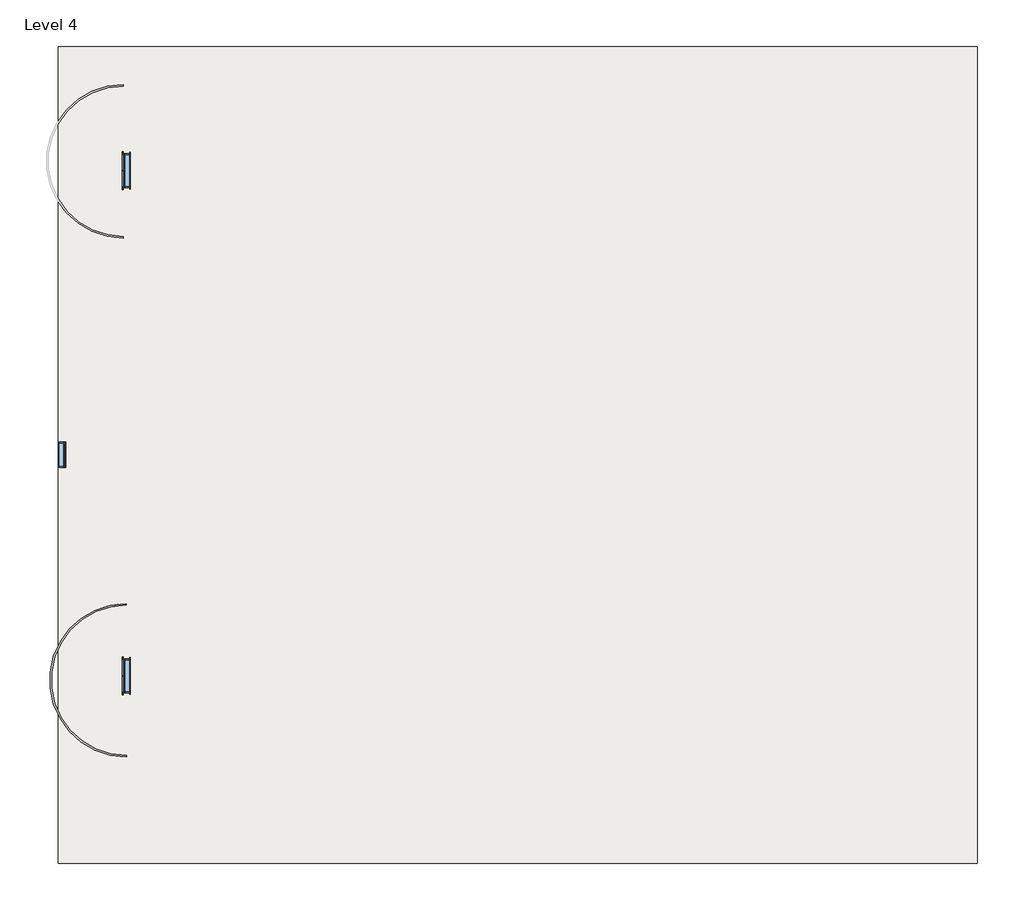
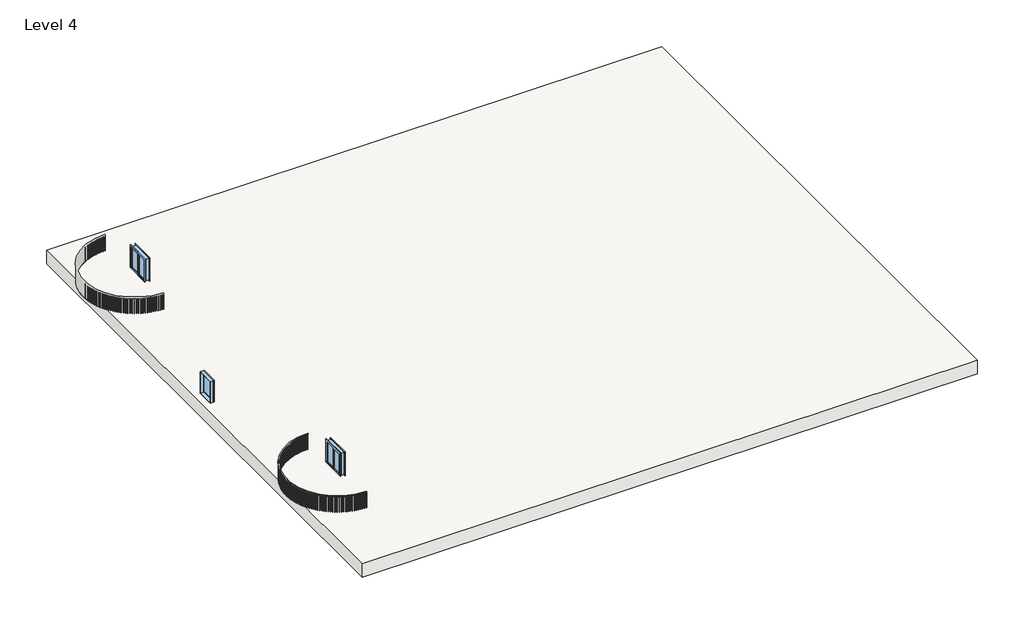
# One storey, part 1 of 2: 3 windows, 1 railing, 1 slab.
"""IFC4 building model written with IfcOpenShell, lengths in millimetres."""

from ifc_helpers import new_model, si_unit, point, frame, frame_2d, origin, place, context, project, spatial, polyline, circle_curve, trimmed, segment, composite_curve, outline, extrude, transform, mapped, element, save
from components import window_534dcd48, window_c1f32544

model = new_model("IFC4")

# Units and contexts
model_context = context("Model", 3, world=origin())
ifc_project = project(units=[si_unit("LENGTHUNIT", "METRE", prefix="MILLI")], contexts=[model_context])

# Site, building, storey
site = spatial("IfcSite", under=ifc_project)
building = spatial("IfcBuilding", under=site)
storey = spatial("IfcBuildingStorey", under=building, Name="Level 4", Elevation=9144.0)

# Railing
placement = place(None, origin())
element("IfcRailing", 1, ObjectType="Handrail - Rectangular", at=placement, inside=storey, context=model_context, shape_type="SweptSolid", body=[
    extrude(outline(composite_curve([segment(trimmed(circle_curve(frame_2d((-15613.8723021, -8267.0443987)), 2743.2), [point((-15613.8723021, -11010.2443987))], [point((-15613.8723021, -5523.8443987))], False, "CARTESIAN"), True, "CONTINUOUS"), segment(polyline([(-15613.8723021, -5523.8443987), (-15613.8723021, -5574.6443987)]), True, "CONTINUOUS"), segment(trimmed(circle_curve(frame_2d((-15613.8723021, -8267.0443987)), 2692.4), [point((-15613.8723021, -5574.6443987))], [point((-15613.8723021, -10959.4443987))], True, "CARTESIAN"), True, "CONTINUOUS"), segment(polyline([(-15613.8723021, -10959.4443987), (-15613.8723021, -11010.2443987)]), True, "CONTINUOUS")], self_intersect=False)), frame((0.0, 0.0, 10007.6), z_axis=(0.0, 0.0, 1.0), x_axis=(1.0, 0.0, 0.0)), (0.0, 0.0, 1.0), 50.8),
    extrude(outline(polyline([(-15627.231195, -10994.3533143), (-15627.2044157, -10975.3033331), (-15608.1544345, -10975.3301124), (-15608.1812138, -10994.3800936), (-15627.231195, -10994.3533143)])), frame((0.0, 0.0, 9144.0), z_axis=(0.0, 0.0, 1.0), x_axis=(1.0, 0.0, 0.0)), (0.0, 0.0, 1.0), 863.6),
    extrude(outline(polyline([(-15729.1535895, -10991.9485449), (-15728.414846, -10972.9128742), (-15709.3791753, -10973.6516178), (-15710.1179188, -10992.6872885), (-15729.1535895, -10991.9485449)])), frame((0.0, 0.0, 9144.0), z_axis=(0.0, 0.0, 1.0), x_axis=(1.0, 0.0, 0.0)), (0.0, 0.0, 1.0), 863.6),
    extrude(outline(polyline([(-15830.914897, -10985.7361601), (-15829.4652214, -10966.7413992), (-15810.4704606, -10968.1910747), (-15811.9201361, -10987.1858356), (-15830.914897, -10985.7361601)])), frame((0.0, 0.0, 9144.0), z_axis=(0.0, 0.0, 1.0), x_axis=(1.0, 0.0, 0.0)), (0.0, 0.0, 1.0), 863.6),
    extrude(outline(polyline([(-15932.3729223, -10975.7248406), (-15930.2143405, -10956.7975316), (-15911.2870315, -10958.9561134), (-15913.4456133, -10977.8834224), (-15932.3729223, -10975.7248406)])), frame((0.0, 0.0, 9144.0), z_axis=(0.0, 0.0, 1.0), x_axis=(1.0, 0.0, 0.0)), (0.0, 0.0, 1.0), 863.6),
    extrude(outline(polyline([(-16033.3858942, -10961.9285757), (-16030.5214224, -10943.0951665), (-16011.6880132, -10945.9596384), (-16014.5524851, -10964.7930475), (-16033.3858942, -10961.9285757)])), frame((0.0, 0.0, 9144.0), z_axis=(0.0, 0.0, 1.0), x_axis=(1.0, 0.0, 0.0)), (0.0, 0.0, 1.0), 863.6),
    extrude(outline(polyline([(-16133.8126634, -10944.3666434), (-16130.2463041, -10925.6534507), (-16111.5331114, -10929.2198099), (-16115.0994706, -10947.9330026), (-16133.8126634, -10944.3666434)])), frame((0.0, 0.0, 9144.0), z_axis=(0.0, 0.0, 1.0), x_axis=(1.0, 0.0, 0.0)), (0.0, 0.0, 1.0), 863.6),
    extrude(outline(polyline([(-16233.5128994, -10923.0635838), (-16229.2496362, -10904.4967562), (-16210.6828086, -10908.7600194), (-16214.9460718, -10927.326847), (-16233.5128994, -10923.0635838)])), frame((0.0, 0.0, 9144.0), z_axis=(0.0, 0.0, 1.0), x_axis=(1.0, 0.0, 0.0)), (0.0, 0.0, 1.0), 863.6),
    extrude(outline(polyline([(-16332.3472874, -10898.0491643), (-16327.3930774, -10879.654646), (-16308.9985591, -10884.608856), (-16313.9527691, -10903.0033743), (-16332.3472874, -10898.0491643)])), frame((0.0, 0.0, 9144.0), z_axis=(0.0, 0.0, 1.0), x_axis=(1.0, 0.0, 0.0)), (0.0, 0.0, 1.0), 863.6),
    extrude(outline(polyline([(-16430.1777221, -10869.3583388), (-16424.5394881, -10851.1618331), (-16406.3429824, -10856.8000671), (-16411.9812164, -10874.9965728), (-16430.1777221, -10869.3583388)])), frame((0.0, 0.0, 9144.0), z_axis=(0.0, 0.0, 1.0), x_axis=(1.0, 0.0, 0.0)), (0.0, 0.0, 1.0), 863.6),
    extrude(outline(polyline([(-16526.8675012, -10837.0311978), (-16520.5531216, -10819.0581316), (-16502.5800554, -10825.3725111), (-16508.8944349, -10843.3455773), (-16526.8675012, -10837.0311978)])), frame((0.0, 0.0, 9144.0), z_axis=(0.0, 0.0, 1.0), x_axis=(1.0, 0.0, 0.0)), (0.0, 0.0, 1.0), 863.6),
    extrude(outline(polyline([(-16622.2815163, -10801.1129136), (-16615.2998146, -10783.3884011), (-16597.5753021, -10790.3701028), (-16604.5570038, -10808.0946153), (-16622.2815163, -10801.1129136)])), frame((0.0, 0.0, 9144.0), z_axis=(0.0, 0.0, 1.0), x_axis=(1.0, 0.0, 0.0)), (0.0, 0.0, 1.0), 863.6),
    extrude(outline(polyline([(-16716.2864416, -10761.653676), (-16708.6471735, -10744.2024845), (-16691.1959821, -10751.8417526), (-16698.8352501, -10769.292944), (-16716.2864416, -10761.653676)])), frame((0.0, 0.0, 9144.0), z_axis=(0.0, 0.0, 1.0), x_axis=(1.0, 0.0, 0.0)), (0.0, 0.0, 1.0), 863.6),
    extrude(outline(polyline([(-16808.7509204, -10718.708623), (-16800.4647607, -10701.5551378), (-16783.3112754, -10709.8412975), (-16791.5974352, -10726.9947828), (-16808.7509204, -10718.708623)])), frame((0.0, 0.0, 9144.0), z_axis=(0.0, 0.0, 1.0), x_axis=(1.0, 0.0, 0.0)), (0.0, 0.0, 1.0), 863.6),
    extrude(outline(polyline([(-16899.5457485, -10672.3377634), (-16890.6242756, -10655.5059536), (-16873.7924658, -10664.4274266), (-16882.7139387, -10681.2592364), (-16899.5457485, -10672.3377634)])), frame((0.0, 0.0, 9144.0), z_axis=(0.0, 0.0, 1.0), x_axis=(1.0, 0.0, 0.0)), (0.0, 0.0, 1.0), 863.6),
    extrude(outline(polyline([(-16988.5440547, -10622.6058931), (-16978.9997349, -10606.1192785), (-16962.5131203, -10615.6635983), (-16972.0574401, -10632.1502129), (-16988.5440547, -10622.6058931)])), frame((0.0, 0.0, 9144.0), z_axis=(0.0, 0.0, 1.0), x_axis=(1.0, 0.0, 0.0)), (0.0, 0.0, 1.0), 863.6),
    extrude(outline(polyline([(-17075.621478, -10569.5825043), (-17065.4676481, -10553.4641223), (-17049.3492661, -10563.6179523), (-17059.5030961, -10579.7363343), (-17075.621478, -10569.5825043)])), frame((0.0, 0.0, 9144.0), z_axis=(0.0, 0.0, 1.0), x_axis=(1.0, 0.0, 0.0)), (0.0, 0.0, 1.0), 863.6),
    extrude(outline(polyline([(-17160.656342, -10513.3416887), (-17149.9071902, -10497.6140622), (-17134.1795637, -10508.363214), (-17144.9287154, -10524.0908405), (-17160.656342, -10513.3416887)])), frame((0.0, 0.0, 9144.0), z_axis=(0.0, 0.0, 1.0), x_axis=(1.0, 0.0, 0.0)), (0.0, 0.0, 1.0), 863.6),
    extrude(outline(polyline([(-17243.5298239, -10453.9620338), (-17232.2003705, -10438.6471396), (-17216.8854763, -10449.976593), (-17228.2149296, -10465.2914872), (-17243.5298239, -10453.9620338)])), frame((0.0, 0.0, 9144.0), z_axis=(0.0, 0.0, 1.0), x_axis=(1.0, 0.0, 0.0)), (0.0, 0.0, 1.0), 863.6),
    extrude(outline(polyline([(-17324.1261214, -10391.5265132), (-17312.2321975, -10376.6457513), (-17297.3514357, -10388.5396752), (-17309.2453596, -10403.4204371), (-17324.1261214, -10391.5265132)])), frame((0.0, 0.0, 9144.0), z_axis=(0.0, 0.0, 1.0), x_axis=(1.0, 0.0, 0.0)), (0.0, 0.0, 1.0), 863.6),
    extrude(outline(polyline([(-17402.3326143, -10326.1223703), (-17389.8908397, -10311.6965343), (-17375.4650036, -10324.1383088), (-17387.9067782, -10338.5641449), (-17402.3326143, -10326.1223703)])), frame((0.0, 0.0, 9144.0), z_axis=(0.0, 0.0, 1.0), x_axis=(1.0, 0.0, 0.0)), (0.0, 0.0, 1.0), 863.6),
    extrude(outline(polyline([(-17478.0400213, -10257.840997), (-17465.0677814, -10243.8902446), (-17451.117029, -10256.8624845), (-17464.0892689, -10270.8132369), (-17478.0400213, -10257.840997)])), frame((0.0, 0.0, 9144.0), z_axis=(0.0, 0.0, 1.0), x_axis=(1.0, 0.0, 0.0)), (0.0, 0.0, 1.0), 863.6),
    extrude(outline(polyline([(-17551.1425537, -10186.7778056), (-17537.6579752, -10173.3216307), (-17524.2018003, -10186.8062093), (-17537.6863789, -10200.2623841), (-17551.1425537, -10186.7778056)])), frame((0.0, 0.0, 9144.0), z_axis=(0.0, 0.0, 1.0), x_axis=(1.0, 0.0, 0.0)), (0.0, 0.0, 1.0), 863.6),
    extrude(outline(polyline([(-17621.5380624, -10113.0320953), (-17607.5599877, -10100.0893009), (-17594.6171933, -10114.0673756), (-17608.595268, -10127.01017), (-17621.5380624, -10113.0320953)])), frame((0.0, 0.0, 9144.0), z_axis=(0.0, 0.0, 1.0), x_axis=(1.0, 0.0, 0.0)), (0.0, 0.0, 1.0), 863.6),
    extrude(outline(polyline([(-17689.128181, -10036.7069141), (-17674.6761422, -10024.2955856), (-17662.2648137, -10038.7476243), (-17676.7168525, -10051.1589528), (-17689.128181, -10036.7069141)])), frame((0.0, 0.0, 9144.0), z_axis=(0.0, 0.0, 1.0), x_axis=(1.0, 0.0, 0.0)), (0.0, 0.0, 1.0), 863.6),
    extrude(outline(polyline([(-17753.8184631, -9957.908914), (-17738.9126547, -9946.0463942), (-17727.0501349, -9960.9522026), (-17741.9559433, -9972.8147224), (-17753.8184631, -9957.908914)])), frame((0.0, 0.0, 9144.0), z_axis=(0.0, 0.0, 1.0), x_axis=(1.0, 0.0, 0.0)), (0.0, 0.0, 1.0), 863.6),
    extrude(outline(polyline([(-17815.5185146, -9876.7482026), (-17800.179765, -9865.4510675), (-17788.8826299, -9880.789817), (-17804.2213795, -9892.0869522), (-17815.5185146, -9876.7482026)])), frame((0.0, 0.0, 9144.0), z_axis=(0.0, 0.0, 1.0), x_axis=(1.0, 0.0, 0.0)), (0.0, 0.0, 1.0), 863.6),
    extrude(outline(polyline([(-17874.1421194, -9793.338189), (-17858.3918621, -9782.6222244), (-17847.6758976, -9798.3724817), (-17863.4261549, -9809.0884462), (-17874.1421194, -9793.338189)])), frame((0.0, 0.0, 9144.0), z_axis=(0.0, 0.0, 1.0), x_axis=(1.0, 0.0, 0.0)), (0.0, 0.0, 1.0), 863.6),
    extrude(outline(polyline([(-17929.6073606, -9707.7954251), (-17913.467604, -9697.6756051), (-17903.347784, -9713.8153616), (-17919.4875405, -9723.9351817), (-17929.6073606, -9707.7954251)])), frame((0.0, 0.0, 9144.0), z_axis=(0.0, 0.0, 1.0), x_axis=(1.0, 0.0, 0.0)), (0.0, 0.0, 1.0), 863.6),
    extrude(outline(polyline([(-17981.8367343, -9620.2394434), (-17965.3300312, -9610.7299086), (-17955.8204964, -9627.2366117), (-17972.3271995, -9636.7461465), (-17981.8367343, -9620.2394434)])), frame((0.0, 0.0, 9144.0), z_axis=(0.0, 0.0, 1.0), x_axis=(1.0, 0.0, 0.0)), (0.0, 0.0, 1.0), 863.6),
    extrude(outline(polyline([(-18030.7572585, -9530.7925891), (-18013.9066743, -9521.9066277), (-18005.0207128, -9538.7572119), (-18021.871297, -9547.6431733), (-18030.7572585, -9530.7925891)])), frame((0.0, 0.0, 9144.0), z_axis=(0.0, 0.0, 1.0), x_axis=(1.0, 0.0, 0.0)), (0.0, 0.0, 1.0), 863.6),
    extrude(outline(polyline([(-18076.3005745, -9439.5798499), (-18059.1296552, -9431.3298785), (-18050.8796837, -9448.5007978), (-18068.0506031, -9456.7507693), (-18076.3005745, -9439.5798499)])), frame((0.0, 0.0, 9144.0), z_axis=(0.0, 0.0, 1.0), x_axis=(1.0, 0.0, 0.0)), (0.0, 0.0, 1.0), 863.6),
    extrude(outline(polyline([(-18118.4030429, -9346.728681), (-18100.9357821, -9339.1262276), (-18093.3333287, -9356.5934885), (-18110.8005895, -9364.1959419), (-18118.4030429, -9346.728681)])), frame((0.0, 0.0, 9144.0), z_axis=(0.0, 0.0, 1.0), x_axis=(1.0, 0.0, 0.0)), (0.0, 0.0, 1.0), 863.6),
    extrude(outline(polyline([(-18157.0058323, -9252.3688268), (-18139.2666376, -9245.4245147), (-18132.3223254, -9263.1637094), (-18150.0615201, -9270.1080215), (-18157.0058323, -9252.3688268)])), frame((0.0, 0.0, 9144.0), z_axis=(0.0, 0.0, 1.0), x_axis=(1.0, 0.0, 0.0)), (0.0, 0.0, 1.0), 863.6),
    extrude(outline(polyline([(-18192.0550015, -9156.6321402), (-18174.0686606, -9150.3556729), (-18167.7921932, -9168.3420137), (-18185.7785341, -9174.6184811), (-18192.0550015, -9156.6321402)])), frame((0.0, 0.0, 9144.0), z_axis=(0.0, 0.0, 1.0), x_axis=(1.0, 0.0, 0.0)), (0.0, 0.0, 1.0), 863.6),
    extrude(outline(polyline([(-18223.5015748, -9059.6523978), (-18205.2932208, -9054.0525456), (-18199.6933686, -9072.2608996), (-18217.9017226, -9077.8607518), (-18223.5015748, -9059.6523978)])), frame((0.0, 0.0, 9144.0), z_axis=(0.0, 0.0, 1.0), x_axis=(1.0, 0.0, 0.0)), (0.0, 0.0, 1.0), 863.6),
    extrude(outline(polyline([(-18251.3016108, -8961.5651131), (-18232.8966869, -8956.6497009), (-18227.9812748, -8975.0546248), (-18246.3861986, -8979.970037), (-18251.3016108, -8961.5651131)])), frame((0.0, 0.0, 9144.0), z_axis=(0.0, 0.0, 1.0), x_axis=(1.0, 0.0, 0.0)), (0.0, 0.0, 1.0), 863.6),
    extrude(outline(polyline([(-18275.4162634, -8862.5073473), (-18256.8404876, -8858.2832437), (-18252.6163839, -8876.8590196), (-18271.1921598, -8881.0831232), (-18275.4162634, -8862.5073473)])), frame((0.0, 0.0, 9144.0), z_axis=(0.0, 0.0, 1.0), x_axis=(1.0, 0.0, 0.0)), (0.0, 0.0, 1.0), 863.6),
    extrude(outline(polyline([(-18295.8118362, -8762.6175179), (-18277.0911651, -8759.0906253), (-18273.5642725, -8777.8112965), (-18292.2849436, -8781.338189), (-18295.8118362, -8762.6175179)])), frame((0.0, 0.0, 9144.0), z_axis=(0.0, 0.0, 1.0), x_axis=(1.0, 0.0, 0.0)), (0.0, 0.0, 1.0), 863.6),
    extrude(outline(polyline([(-18312.4598298, -8662.0352047), (-18293.6204224, -8659.2104514), (-18290.7956691, -8678.0498587), (-18309.6350765, -8680.874612), (-18312.4598298, -8662.0352047)])), frame((0.0, 0.0, 9144.0), z_axis=(0.0, 0.0, 1.0), x_axis=(1.0, 0.0, 0.0)), (0.0, 0.0, 1.0), 863.6),
    extrude(outline(polyline([(-18325.3369811, -8560.9009553), (-18306.4051626, -8558.7822885), (-18304.2864958, -8577.714107), (-18323.2183143, -8579.8327738), (-18325.3369811, -8560.9009553)])), frame((0.0, 0.0, 9144.0), z_axis=(0.0, 0.0, 1.0), x_axis=(1.0, 0.0, 0.0)), (0.0, 0.0, 1.0), 863.6),
    extrude(outline(polyline([(-18334.4252965, -8459.3560886), (-18315.427521, -8457.9464688), (-18314.0179011, -8476.9442442), (-18333.0156766, -8478.3538641), (-18334.4252965, -8459.3560886)])), frame((0.0, 0.0, 9144.0), z_axis=(0.0, 0.0, 1.0), x_axis=(1.0, 0.0, 0.0)), (0.0, 0.0, 1.0), 863.6),
    extrude(outline(polyline([(-18339.7120764, -8357.5424973), (-18320.6748904, -8356.8438941), (-18319.9762872, -8375.8810802), (-18339.0134732, -8376.5796834), (-18339.7120764, -8357.5424973)])), frame((0.0, 0.0, 9144.0), z_axis=(0.0, 0.0, 1.0), x_axis=(1.0, 0.0, 0.0)), (0.0, 0.0, 1.0), 863.6),
    extrude(outline(polyline([(-18341.1899336, -8255.6024494), (-18322.1399383, -8255.6158391), (-18322.1533279, -8274.6658344), (-18341.2033232, -8274.6524447), (-18341.1899336, -8255.6024494)])), frame((0.0, 0.0, 9144.0), z_axis=(0.0, 0.0, 1.0), x_axis=(1.0, 0.0, 0.0)), (0.0, 0.0, 1.0), 863.6),
    extrude(outline(polyline([(-18338.8568028, -8153.6783898), (-18319.8206176, -8154.4037536), (-18320.5459814, -8173.4399388), (-18339.5821666, -8172.7145751), (-18338.8568028, -8153.6783898)])), frame((0.0, 0.0, 9144.0), z_axis=(0.0, 0.0, 1.0), x_axis=(1.0, 0.0, 0.0)), (0.0, 0.0, 1.0), 863.6),
    extrude(outline(polyline([(-18332.7159444, -8051.912741), (-18313.7201692, -8053.3490654), (-18315.1564936, -8072.3448405), (-18334.1522687, -8070.9085161), (-18332.7159444, -8051.912741)])), frame((0.0, 0.0, 9144.0), z_axis=(0.0, 0.0, 1.0), x_axis=(1.0, 0.0, 0.0)), (0.0, 0.0, 1.0), 863.6),
    extrude(outline(polyline([(-18322.775939, -7950.4477041), (-18303.8471175, -7952.592982), (-18305.9923954, -7971.5218035), (-18324.9212169, -7969.3765256), (-18322.775939, -7950.4477041)])), frame((0.0, 0.0, 9144.0), z_axis=(0.0, 0.0, 1.0), x_axis=(1.0, 0.0, 0.0)), (0.0, 0.0, 1.0), 863.6),
    extrude(outline(polyline([(-18309.0506764, -7849.4250602), (-18290.2152585, -7852.2762939), (-18293.0664923, -7871.1117118), (-18311.9019101, -7868.260478), (-18309.0506764, -7849.4250602)])), frame((0.0, 0.0, 9144.0), z_axis=(0.0, 0.0, 1.0), x_axis=(1.0, 0.0, 0.0)), (0.0, 0.0, 1.0), 863.6),
    extrude(outline(polyline([(-18291.5593353, -7748.9859721), (-18272.8436405, -7752.5391776), (-18276.396846, -7771.2548723), (-18295.1125408, -7767.7016669), (-18291.5593353, -7748.9859721)])), frame((0.0, 0.0, 9144.0), z_axis=(0.0, 0.0, 1.0), x_axis=(1.0, 0.0, 0.0)), (0.0, 0.0, 1.0), 863.6),
    extrude(outline(polyline([(-18270.3263571, -7649.2707874), (-18251.7565376, -7653.5209995), (-18256.0067497, -7672.0908191), (-18274.5765692, -7667.8406069), (-18270.3263571, -7649.2707874)])), frame((0.0, 0.0, 9144.0), z_axis=(0.0, 0.0, 1.0), x_axis=(1.0, 0.0, 0.0)), (0.0, 0.0, 1.0), 863.6),
    extrude(outline(polyline([(-18245.3814115, -7550.418842), (-18226.9834156, -7555.3601218), (-18231.9246954, -7573.7581178), (-18250.3226913, -7568.816838), (-18245.3814115, -7550.418842)])), frame((0.0, 0.0, 9144.0), z_axis=(0.0, 0.0, 1.0), x_axis=(1.0, 0.0, 0.0)), (0.0, 0.0, 1.0), 863.6),
    extrude(outline(polyline([(-18216.7593549, -7452.5682656), (-18198.5588909, -7458.1937085), (-18204.1843337, -7476.3941726), (-18222.3847978, -7470.7687297), (-18216.7593549, -7452.5682656)])), frame((0.0, 0.0, 9144.0), z_axis=(0.0, 0.0, 1.0), x_axis=(1.0, 0.0, 0.0)), (0.0, 0.0, 1.0), 863.6),
    extrude(outline(polyline([(-18184.5001822, -7355.8557887), (-18166.5226822, -7362.1575339), (-18172.8244275, -7380.1350339), (-18190.8019275, -7373.8332887), (-18184.5001822, -7355.8557887)])), frame((0.0, 0.0, 9144.0), z_axis=(0.0, 0.0, 1.0), x_axis=(1.0, 0.0, 0.0)), (0.0, 0.0, 1.0), 863.6),
    extrude(outline(polyline([(-18148.6489704, -7260.4165513), (-18130.9195551, -7267.3857933), (-18137.888797, -7285.1152086), (-18155.6182123, -7278.1459666), (-18148.6489704, -7260.4165513)])), frame((0.0, 0.0, 9144.0), z_axis=(0.0, 0.0, 1.0), x_axis=(1.0, 0.0, 0.0)), (0.0, 0.0, 1.0), 863.6),
    extrude(outline(polyline([(-18109.2558157, -7166.3839145), (-18091.7992591, -7174.0109148), (-18099.4262594, -7191.4674713), (-18116.8828159, -7183.8404711), (-18109.2558157, -7166.3839145)])), frame((0.0, 0.0, 9144.0), z_axis=(0.0, 0.0, 1.0), x_axis=(1.0, 0.0, 0.0)), (0.0, 0.0, 1.0), 863.6),
    extrude(outline(polyline([(-18066.3757637, -7073.8892738), (-18049.2164586, -7082.1633749), (-18057.4905597, -7099.32268), (-18074.6498648, -7091.0485789), (-18066.3757637, -7073.8892738)])), frame((0.0, 0.0, 9144.0), z_axis=(0.0, 0.0, 1.0), x_axis=(1.0, 0.0, 0.0)), (0.0, 0.0, 1.0), 863.6),
    extrude(outline(polyline([(-18020.0687324, -6983.0618755), (-18003.2306562, -6991.9715157), (-18012.1402963, -7008.8095919), (-18028.9783726, -6999.8999518), (-18020.0687324, -6983.0618755)])), frame((0.0, 0.0, 9144.0), z_axis=(0.0, 0.0, 1.0), x_axis=(1.0, 0.0, 0.0)), (0.0, 0.0, 1.0), 863.6),
    extrude(outline(polyline([(-17970.3994285, -6894.0286364), (-17953.9061096, -6903.5613658), (-17963.4388391, -6920.0546848), (-17979.932158, -6910.5219553), (-17970.3994285, -6894.0286364)])), frame((0.0, 0.0, 9144.0), z_axis=(0.0, 0.0, 1.0), x_axis=(1.0, 0.0, 0.0)), (0.0, 0.0, 1.0), 863.6),
    extrude(outline(polyline([(-17917.4372568, -6806.913966), (-17901.311742, -6817.0564643), (-17911.4542403, -6833.1819791), (-17927.5797552, -6823.0394808), (-17917.4372568, -6806.913966)])), frame((0.0, 0.0, 9144.0), z_axis=(0.0, 0.0, 1.0), x_axis=(1.0, 0.0, 0.0)), (0.0, 0.0, 1.0), 863.6),
    extrude(outline(polyline([(-17861.2562235, -6721.8395932), (-17845.5210456, -6732.5776878), (-17856.2591402, -6748.3128657), (-17871.9943181, -6737.5747711), (-17861.2562235, -6721.8395932)])), frame((0.0, 0.0, 9144.0), z_axis=(0.0, 0.0, 1.0), x_axis=(1.0, 0.0, 0.0)), (0.0, 0.0, 1.0), 863.6),
    extrude(outline(polyline([(-17801.9348324, -6638.9243956), (-17786.6119788, -6650.2430818), (-17797.9306651, -6665.5659354), (-17813.2535187, -6654.2472492), (-17801.9348324, -6638.9243956)])), frame((0.0, 0.0, 9144.0), z_axis=(0.0, 0.0, 1.0), x_axis=(1.0, 0.0, 0.0)), (0.0, 0.0, 1.0), 863.6),
    extrude(outline(polyline([(-17739.5559758, -6558.284234), (-17724.6668577, -6570.1676957), (-17736.5503195, -6585.0568138), (-17751.4394375, -6573.1733521), (-17739.5559758, -6558.284234)])), frame((0.0, 0.0, 9144.0), z_axis=(0.0, 0.0, 1.0), x_axis=(1.0, 0.0, 0.0)), (0.0, 0.0, 1.0), 863.6),
    extrude(outline(polyline([(-17674.206818, -6480.03179), (-17659.7722406, -6492.463422), (-17672.2038726, -6506.8979994), (-17686.63845, -6494.4663674), (-17674.206818, -6480.03179)])), frame((0.0, 0.0, 9144.0), z_axis=(0.0, 0.0, 1.0), x_axis=(1.0, 0.0, 0.0)), (0.0, 0.0, 1.0), 863.6),
    extrude(outline(polyline([(-17605.978674, -6404.2764087), (-17592.0188072, -6417.2388399), (-17604.9812384, -6431.1987066), (-17618.9411051, -6418.2362755), (-17605.978674, -6404.2764087)])), frame((0.0, 0.0, 9144.0), z_axis=(0.0, 0.0, 1.0), x_axis=(1.0, 0.0, 0.0)), (0.0, 0.0, 1.0), 863.6),
    extrude(outline(polyline([(-17534.9668816, -6331.1239463), (-17521.5012322, -6344.5990636), (-17534.9763495, -6358.064713), (-17548.4419989, -6344.5895957), (-17534.9668816, -6331.1239463)])), frame((0.0, 0.0, 9144.0), z_axis=(0.0, 0.0, 1.0), x_axis=(1.0, 0.0, 0.0)), (0.0, 0.0, 1.0), 863.6),
    extrude(outline(polyline([(-17461.2706683, -6260.6766214), (-17448.3180524, -6274.6455956), (-17462.2870265, -6287.5982116), (-17475.2396425, -6273.6292374), (-17461.2706683, -6260.6766214)])), frame((0.0, 0.0, 9144.0), z_axis=(0.0, 0.0, 1.0), x_axis=(1.0, 0.0, 0.0)), (0.0, 0.0, 1.0), 863.6),
    extrude(outline(polyline([(-17384.9930129, -6193.032873), (-17372.5715296, -6207.4761846), (-17387.0148412, -6219.897668), (-17399.4363246, -6205.4543563), (-17384.9930129, -6193.032873)])), frame((0.0, 0.0, 9144.0), z_axis=(0.0, 0.0, 1.0), x_axis=(1.0, 0.0, 0.0)), (0.0, 0.0, 1.0), 863.6),
    extrude(outline(polyline([(-17306.2405011, -6128.2872222), (-17294.3675074, -6143.1846891), (-17309.2649743, -6155.0576828), (-17321.137968, -6140.1602159), (-17306.2405011, -6128.2872222)])), frame((0.0, 0.0, 9144.0), z_axis=(0.0, 0.0, 1.0), x_axis=(1.0, 0.0, 0.0)), (0.0, 0.0, 1.0), 863.6),
    extrude(outline(polyline([(-17225.1231768, -6066.5301406), (-17213.8152633, -6081.860946), (-17229.1460687, -6093.1688594), (-17240.4539822, -6077.8380541), (-17225.1231768, -6066.5301406)])), frame((0.0, 0.0, 9144.0), z_axis=(0.0, 0.0, 1.0), x_axis=(1.0, 0.0, 0.0)), (0.0, 0.0, 1.0), 863.6),
    extrude(outline(polyline([(-17141.7543884, -6007.847924), (-17131.0273562, -6023.5906455), (-17146.7700777, -6034.3176777), (-17157.4971099, -6018.5749562), (-17141.7543884, -6007.847924)])), frame((0.0, 0.0, 9144.0), z_axis=(0.0, 0.0, 1.0), x_axis=(1.0, 0.0, 0.0)), (0.0, 0.0, 1.0), 863.6),
    extrude(outline(polyline([(-17056.2506305, -5952.3225712), (-17046.1194688, -5968.4552108), (-17062.2521085, -5978.5863725), (-17072.3832702, -5962.4537328), (-17056.2506305, -5952.3225712)])), frame((0.0, 0.0, 9144.0), z_axis=(0.0, 0.0, 1.0), x_axis=(1.0, 0.0, 0.0)), (0.0, 0.0, 1.0), 863.6),
    extrude(outline(polyline([(-16968.7313808, -5900.03167), (-16959.2102463, -5916.5316851), (-16975.7102614, -5926.0528195), (-16985.2313959, -5909.5528044), (-16968.7313808, -5900.03167)])), frame((0.0, 0.0, 9144.0), z_axis=(0.0, 0.0, 1.0), x_axis=(1.0, 0.0, 0.0)), (0.0, 0.0, 1.0), 863.6),
    extrude(outline(polyline([(-16879.3189333, -5851.0482885), (-16870.4211303, -5867.8926229), (-16887.2654647, -5876.7904259), (-16896.1632677, -5859.9460915), (-16879.3189333, -5851.0482885)])), frame((0.0, 0.0, 9144.0), z_axis=(0.0, 0.0, 1.0), x_axis=(1.0, 0.0, 0.0)), (0.0, 0.0, 1.0), 863.6),
    extrude(outline(polyline([(-16788.1382277, -5805.4408731), (-16779.8761894, -5822.6059896), (-16797.0413058, -5830.8680279), (-16805.3033441, -5813.7029114), (-16788.1382277, -5805.4408731)])), frame((0.0, 0.0, 9144.0), z_axis=(0.0, 0.0, 1.0), x_axis=(1.0, 0.0, 0.0)), (0.0, 0.0, 1.0), 863.6),
    extrude(outline(polyline([(-16695.3166742, -5763.2731529), (-16687.7019455, -5780.7350659), (-16705.1638585, -5788.3497946), (-16712.7785872, -5770.8878816), (-16695.3166742, -5763.2731529)])), frame((0.0, 0.0, 9144.0), z_axis=(0.0, 0.0, 1.0), x_axis=(1.0, 0.0, 0.0)), (0.0, 0.0, 1.0), 863.6),
    extrude(outline(polyline([(-16600.983976, -5724.6040505), (-16594.0271973, -5742.3383598), (-16611.7615066, -5749.2951386), (-16618.7182854, -5731.5608292), (-16600.983976, -5724.6040505)])), frame((0.0, 0.0, 9144.0), z_axis=(0.0, 0.0, 1.0), x_axis=(1.0, 0.0, 0.0)), (0.0, 0.0, 1.0), 863.6),
    extrude(outline(polyline([(-16505.271948, -5689.4875996), (-16498.9828402, -5707.4695245), (-16516.9647651, -5713.7586324), (-16523.2538729, -5695.7767075), (-16505.271948, -5689.4875996)])), frame((0.0, 0.0, 9144.0), z_axis=(0.0, 0.0, 1.0), x_axis=(1.0, 0.0, 0.0)), (0.0, 0.0, 1.0), 863.6),
    extrude(outline(polyline([(-16408.3143324, -5657.97287), (-16402.7016834, -5676.1772836), (-16420.906097, -5681.7899325), (-16426.5187459, -5663.5855189), (-16408.3143324, -5657.97287)])), frame((0.0, 0.0, 9144.0), z_axis=(0.0, 0.0, 1.0), x_axis=(1.0, 0.0, 0.0)), (0.0, 0.0, 1.0), 863.6),
    extrude(outline(polyline([(-16310.2466117, -5630.1038984), (-16305.3182645, -5648.5053628), (-16323.7197289, -5653.43371), (-16328.6480761, -5635.0322456), (-16310.2466117, -5630.1038984)])), frame((0.0, 0.0, 9144.0), z_axis=(0.0, 0.0, 1.0), x_axis=(1.0, 0.0, 0.0)), (0.0, 0.0, 1.0), 863.6),
    extrude(outline(polyline([(-16211.2058198, -5605.9196271), (-16206.9686609, -5624.4924294), (-16225.5414632, -5628.7295883), (-16229.7786221, -5610.1567861), (-16211.2058198, -5605.9196271)])), frame((0.0, 0.0, 9144.0), z_axis=(0.0, 0.0, 1.0), x_axis=(1.0, 0.0, 0.0)), (0.0, 0.0, 1.0), 863.6),
    extrude(outline(polyline([(-16111.3303505, -5585.4538499), (-16107.7903006, -5604.1720375), (-16126.5084882, -5607.7120874), (-16130.048538, -5588.9938998), (-16111.3303505, -5585.4538499)])), frame((0.0, 0.0, 9144.0), z_axis=(0.0, 0.0, 1.0), x_axis=(1.0, 0.0, 0.0)), (0.0, 0.0, 1.0), 863.6),
    extrude(outline(polyline([(-16010.7597634, -5568.7351643), (-16007.9217692, -5587.5725816), (-16026.7591865, -5590.4105758), (-16029.5971807, -5571.5731585), (-16010.7597634, -5568.7351643)])), frame((0.0, 0.0, 9144.0), z_axis=(0.0, 0.0, 1.0), x_axis=(1.0, 0.0, 0.0)), (0.0, 0.0, 1.0), 863.6),
    extrude(outline(polyline([(-15909.63459, -5555.7869321), (-15907.5026171, -5574.7172567), (-15926.4329418, -5576.8492296), (-15928.5649146, -5557.918905), (-15909.63459, -5555.7869321)])), frame((0.0, 0.0, 9144.0), z_axis=(0.0, 0.0, 1.0), x_axis=(1.0, 0.0, 0.0)), (0.0, 0.0, 1.0), 863.6),
    extrude(outline(polyline([(-15808.0961363, -5546.6272462), (-15806.6731638, -5565.6240262), (-15825.6699438, -5567.0469987), (-15827.0929163, -5548.0502187), (-15808.0961363, -5546.6272462)])), frame((0.0, 0.0, 9144.0), z_axis=(0.0, 0.0, 1.0), x_axis=(1.0, 0.0, 0.0)), (0.0, 0.0, 1.0), 863.6),
    extrude(outline(polyline([(-15706.286286, -5541.268906), (-15705.5743024, -5560.3055963), (-15724.6109927, -5561.01758), (-15725.3229764, -5541.9808896), (-15706.286286, -5541.268906)])), frame((0.0, 0.0, 9144.0), z_axis=(0.0, 0.0, 1.0), x_axis=(1.0, 0.0, 0.0)), (0.0, 0.0, 1.0), 863.6),
    extrude(outline(polyline([(-15632.955606, -10994.3192673), (-15632.8888422, -10975.2693843), (-15613.8389591, -10975.3361482), (-15613.905723, -10994.3860312), (-15632.955606, -10994.3192673)])), frame((0.0, 0.0, 9144.0), z_axis=(0.0, 0.0, 1.0), x_axis=(1.0, 0.0, 0.0)), (0.0, 0.0, 1.0), 863.6),
    extrude(outline(polyline([(-15613.905723, -5539.7027662), (-15613.8389591, -5558.7526493), (-15632.8888422, -5558.8194131), (-15632.955606, -5539.7695301), (-15613.905723, -5539.7027662)])), frame((0.0, 0.0, 9144.0), z_axis=(0.0, 0.0, 1.0), x_axis=(1.0, 0.0, 0.0)), (0.0, 0.0, 1.0), 863.6),
])

# Slab
element("IfcSlab", 2, ObjectType="Generic - 12\"", at=placement, inside=storey, context=model_context, shape_type="SweptSolid", body=[
    extrude(outline(polyline([(14866.1276979, 14440.5556013), (14866.1276979, -14820.2443987), (-18052.2723021, -14820.2443987), (-18052.2723021, 14440.5556013), (14866.1276979, 14440.5556013)])), frame((0.0, 0.0, 8382.0), z_axis=(0.0, 0.0, 1.0), x_axis=(1.0, 0.0, 0.0)), (0.0, 0.0, 1.0), 762.0),
])

# Windows
window_shape = window_534dcd48(model_context)
element("IfcWindow", 3, ObjectType="Casement Dbl with Trim : 48\" x 48\"", at=placement, inside=storey, context=model_context, shape_type="MappedRepresentation", body=[
    mapped(window_shape, transform((-15594.8223021, 9995.5556013, 8737.1054136), x_axis=(0.0, 1.0, 0.0), y_axis=(-1.0, 0.0, 0.0), z_axis=(0.0, 0.0, 1.0))),
])
element("IfcWindow", 4, ObjectType="Casement Dbl with Trim : 48\" x 48\"", at=placement, inside=storey, context=model_context, shape_type="MappedRepresentation", body=[
    mapped(window_shape, transform((-15594.8223021, -8114.6443987, 8725.1499872), x_axis=(0.0, 1.0, 0.0), y_axis=(-1.0, 0.0, 0.0), z_axis=(0.0, 0.0, 1.0))),
])
window_2_shape = window_c1f32544(model_context)
element("IfcWindow", 5, ObjectType="Fixed : 36\" x 48\"", at=placement, inside=storey, context=model_context, shape_type="MappedRepresentation", body=[
    mapped(window_2_shape, transform((-17899.8723021, -227.9443987, 8721.0470019), x_axis=(0.0, -1.0, 0.0), y_axis=(1.0, 0.0, 0.0), z_axis=(0.0, 0.0, 1.0))),
])

save(model, "model.ifc")

# Revit data of these elements
# Type "Handrail - Rectangular"
#   Assembly Code = "C2010400"
#   built-in parameter 1008612 = 0.0416667 (stored number, unit not read)
#   built-in parameter 1008611 = 0.0416667 (stored number, unit not read)
#   built-in parameter 1008609 = 0.333333 (stored number, unit not read)
#   built-in parameter 1008604 = 0.166667 (stored number, unit not read)
#   built-in parameter 1008603 = 0.166667 (stored number, unit not read)
#   Railing Height = 3' - 0"
#   built-in parameter 1008630 = 2
#   built-in parameter 1008610 = 2
#   built-in parameter 1008618 = Baluster - Square : 3/4"
# Type "Generic - 12\""
#   Assembly Code = "B1010"
#   Function = 0
#   Layers, outside or top first: 2' - 6" no material (function 1)
# Type "Casement Dbl with Trim : 48\" x 48\""
#   Type Mark = "19"
#   Construction Type Id = "GSP4R"
#   Assembly Code = "B2020100"
#   Analytic Construction = "1/8 in Pilkington single glazing"
#   Visual Light Transmittance = 0.9
#   Solar Heat Gain Coefficient = 0.78
#   Heat Transfer Coefficient (U) = 0.6496 BTU/(h·ft²·°F)
#   Height = 4' - 0"
#   Default Sill Height = 3' - 0"
#   Trim Projection - Ext. = 0' - 0 1/2"
#   Trim Projection - Int. = 0' - 0 3/4"
#   Trim Width - Exterior = 0' - 3 1/2"
#   Trim Width - Interior = 0' - 3 1/2"
#   Width = 4' - 0"
#   Window Inset = 0' - 0 3/4"
#   Define Thermal Properties by = 1
#   Glass Pane Material = Glass
#   Sash Material = Sash
#   Trim Exterior Material = Trim
#   Trim Interior Material = Trim
#   Wall Closure = (empty or 0)
# Type "Fixed : 36\" x 48\""
#   Type Mark = "1"
#   Construction Type Id = "GSP4R"
#   Assembly Code = "B2020100"
#   Analytic Construction = "1/8 in Pilkington single glazing"
#   Visual Light Transmittance = 0.9
#   Solar Heat Gain Coefficient = 0.78
#   Heat Transfer Coefficient (U) = 0.6496 BTU/(h·ft²·°F)
#   Height = 4' - 0"
#   Default Sill Height = 3' - 0"
#   Width = 3' - 0"
#   Window Inset = 0' - 0 3/4"
#   Define Thermal Properties by = 1
#   Glass Pane Material = Glass
#   Sash Material = Sash
#   Wall Closure = (empty or 0)
# Element 1 (IfcRailing, "Handrail - Rectangular")
#   Phase Created = New Construction
# Element 2 (IfcSlab, "Generic - 12\"")
#   Height Offset From Level = 0' - 0"
#   Phase Created = New Construction
#   Materials on its faces: "Default Floor"
# Element 3 (IfcWindow, "Casement Dbl with Trim : 48\" x 48\"")
#   Mark = "8"
#   Phase Created = New Construction
#   Materials on its faces: "Sash", "Trim", "Glass"
# Element 4 (IfcWindow, "Casement Dbl with Trim : 48\" x 48\"")
#   Mark = "11"
#   Phase Created = New Construction
#   Materials on its faces: "Sash", "Trim", "Glass"
# Element 5 (IfcWindow, "Fixed : 36\" x 48\"")
#   Mark = "21"
#   Phase Created = New Construction
#   Materials on its faces: "Sash", "Glass"
# Materials
#   "Glass": class "Glass", colour RGB 0 128 192, transparency 0.75, Description = "Soda Lime Glass", Cost = 0
#   "Sash": class "Wood", colour RGB 224 178 126, transparency 0
#   "Trim": class "Wood", colour RGB 224 178 126, transparency 0
#   "Default Floor": colour RGB 128 128 128, transparency 0
